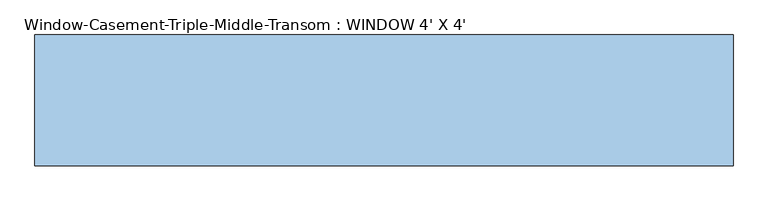
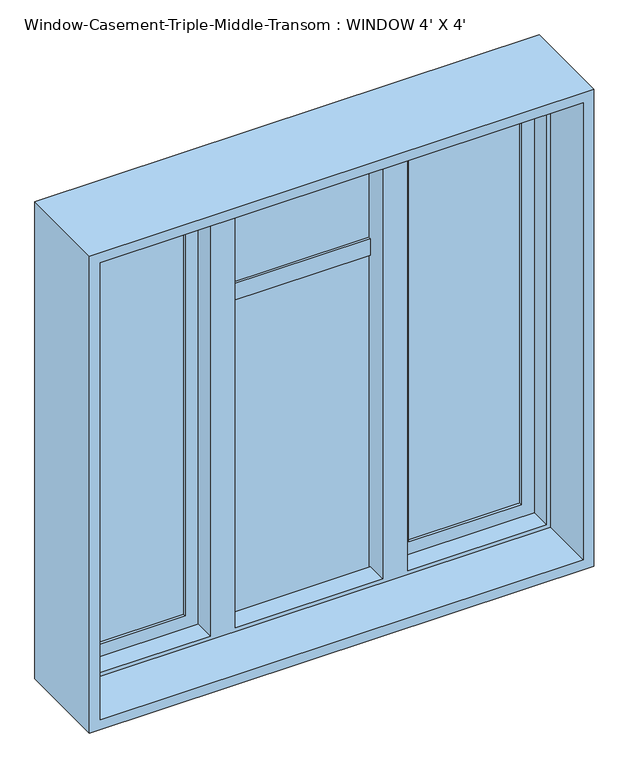
"""IFC4 building model written with IfcOpenShell, lengths in millimetres: window geometry, Window-Casement-Triple-Middle-Transom : WINDOW 4' X 4'."""

from ifc_helpers import new_model, si_unit, frame, origin, place, context, project, spatial, polyline, outline, extrude, faceted_brep, source, transform, mapped, element, save


def window_casement_triple_middle_transom_window_4_x_4_1416bf83(model_context):
    return source(origin(), model_context, "Body", "SolidModel", [
        extrude(outline(polyline([(2108.2, 228.6), (939.8, 228.6), (939.8, 584.2), (2108.2, 584.2), (2108.2, 228.6)]), holes=[polyline([(2066.3296875, 542.3296875), (981.6703125, 542.3296875), (981.6703125, 270.4703125), (2066.3296875, 270.4703125), (2066.3296875, 542.3296875)])]), frame((0.0, 73.025, 0.0), z_axis=(0.0, 1.0, 0.0), x_axis=(0.0, 0.0, 1.0)), (0.0, 0.0, 1.0), 31.75),
        extrude(outline(polyline([(2108.2, -584.2), (939.8, -584.2), (939.8, -228.6), (2108.2, -228.6), (2108.2, -584.2)]), holes=[polyline([(2066.3296875, -270.4703125), (981.6703125, -270.4703125), (981.6703125, -542.3296875), (2066.3296875, -542.3296875), (2066.3296875, -270.4703125)])]), frame((0.0, 73.025, 0.0), z_axis=(0.0, 1.0, 0.0), x_axis=(0.0, 0.0, 1.0)), (0.0, 0.0, 1.0), 31.75),
        extrude(outline(polyline([(-270.4703125, 98.425), (-270.4703125, 92.075), (-542.3296875, 92.075), (-542.3296875, 98.425), (-270.4703125, 98.425)])), frame((0.0, 0.0, 949.9203125), z_axis=(0.0, 0.0, 1.0), x_axis=(1.0, 0.0, 0.0)), (0.0, 0.0, 1.0), 1148.159375),
        extrude(outline(polyline([(-270.4703125, 85.725), (-270.4703125, 79.375), (-542.3296875, 79.375), (-542.3296875, 85.725), (-270.4703125, 85.725)])), frame((0.0, 0.0, 949.9203125), z_axis=(0.0, 0.0, 1.0), x_axis=(1.0, 0.0, 0.0)), (0.0, 0.0, 1.0), 1148.159375),
        extrude(outline(polyline([(542.3296875, 98.425), (542.3296875, 92.075), (270.4703125, 92.075), (270.4703125, 98.425), (542.3296875, 98.425)])), frame((0.0, 0.0, 949.9203125), z_axis=(0.0, 0.0, 1.0), x_axis=(1.0, 0.0, 0.0)), (0.0, 0.0, 1.0), 1148.159375),
        extrude(outline(polyline([(542.3296875, 85.725), (542.3296875, 79.375), (270.4703125, 79.375), (270.4703125, 85.725), (542.3296875, 85.725)])), frame((0.0, 0.0, 949.9203125), z_axis=(0.0, 0.0, 1.0), x_axis=(1.0, 0.0, 0.0)), (0.0, 0.0, 1.0), 1148.159375),
        extrude(outline(polyline([(177.8, 104.775), (177.8, 73.025), (-177.8, 73.025), (-177.8, 104.775), (177.8, 104.775)])), frame((0.0, 0.0, 1746.9048438), z_axis=(0.0, 0.0, 1.0), x_axis=(1.0, 0.0, 0.0)), (0.0, 0.0, 1.0), 41.8703125),
        extrude(outline(polyline([(177.8, 98.425), (177.8, 92.075), (-177.8, 92.075), (-177.8, 98.425), (177.8, 98.425)])), frame((0.0, 0.0, 939.8), z_axis=(0.0, 0.0, 1.0), x_axis=(1.0, 0.0, 0.0)), (0.0, 0.0, 1.0), 807.1048438),
        extrude(outline(polyline([(177.8, 85.725), (177.8, 79.375), (-177.8, 79.375), (-177.8, 85.725), (177.8, 85.725)])), frame((0.0, 0.0, 939.8), z_axis=(0.0, 0.0, 1.0), x_axis=(1.0, 0.0, 0.0)), (0.0, 0.0, 1.0), 807.1048438),
        extrude(outline(polyline([(177.8, 98.425), (177.8, 92.075), (-177.8, 92.075), (-177.8, 98.425), (177.8, 98.425)])), frame((0.0, 0.0, 1788.7751563), z_axis=(0.0, 0.0, 1.0), x_axis=(1.0, 0.0, 0.0)), (0.0, 0.0, 1.0), 319.4248438),
        extrude(outline(polyline([(177.8, 85.725), (177.8, 79.375), (-177.8, 79.375), (-177.8, 85.725), (177.8, 85.725)])), frame((0.0, 0.0, 1788.7751563), z_axis=(0.0, 0.0, 1.0), x_axis=(1.0, 0.0, 0.0)), (0.0, 0.0, 1.0), 319.4248438),
        faceted_brep([(-228.6, 73.025, 2108.2), (-584.2, 73.025, 2108.2), (-584.2, 114.3, 2108.2), (584.2, 114.3, 2108.2), (584.2, 73.025, 2108.2), (228.6, 73.025, 2108.2), (228.6, 111.125, 2108.2), (177.8, 111.125, 2108.2), (177.8, 73.025, 2108.2), (-177.8, 73.025, 2108.2), (-177.8, 111.125, 2108.2), (-228.6, 111.125, 2108.2), (-574.0796875, 22.225, 2098.0796875), (-574.0796875, 73.025, 2098.0796875), (-238.7203125, 73.025, 2098.0796875), (-238.7203125, 22.225, 2098.0796875), (574.0796875, 73.025, 2098.0796875), (574.0796875, 22.225, 2098.0796875), (238.7203125, 22.225, 2098.0796875), (238.7203125, 73.025, 2098.0796875), (-177.8, 73.025, 2098.0796875), (177.8, 73.025, 2098.0796875), (177.8, 22.225, 2098.0796875), (-177.8, 22.225, 2098.0796875), (-584.2, -114.3, 2108.2), (-584.2, 22.225, 2108.2), (584.2, 22.225, 2108.2), (584.2, -114.3, 2108.2), (-609.6, 114.3, 2133.6), (-609.6, -114.3, 2133.6), (609.6, -114.3, 2133.6), (609.6, 114.3, 2133.6), (584.2, 114.3, 939.8), (584.2, 73.025, 939.8), (574.0796875, 73.025, 949.9203125), (574.0796875, 22.225, 949.9203125), (584.2, 22.225, 939.8), (584.2, -114.3, 939.8), (609.6, -114.3, 914.4), (609.6, 114.3, 914.4), (228.6, 73.025, 939.8), (-584.2, 114.3, 939.8), (-584.2, 73.025, 939.8), (-228.6, 73.025, 939.8), (-228.6, 111.125, 939.8), (-177.8, 111.125, 939.8), (-177.8, 73.025, 939.8), (177.8, 73.025, 939.8), (177.8, 111.125, 939.8), (228.6, 111.125, 939.8), (238.7203125, 73.025, 949.9203125), (238.7203125, 22.225, 949.9203125), (-574.0796875, 73.025, 949.9203125), (-574.0796875, 22.225, 949.9203125), (-238.7203125, 22.225, 949.9203125), (-238.7203125, 73.025, 949.9203125), (177.8, 73.025, 949.9203125), (-177.8, 73.025, 949.9203125), (-177.8, 22.225, 949.9203125), (177.8, 22.225, 949.9203125), (-584.2, 22.225, 939.8), (-584.2, -114.3, 939.8), (-609.6, -114.3, 914.4), (-609.6, 114.3, 914.4)], [[[0, 1, 2, 3, 4, 5, 6, 7, 8, 9, 10, 11]], [[12, 13, 14, 15]], [[16, 17, 18, 19]], [[20, 21, 22, 23]], [[24, 25, 26, 27]], [[28, 29, 30, 31]], [[4, 3, 32, 33]], [[17, 16, 34, 35]], [[27, 26, 36, 37]], [[31, 30, 38, 39]], [[40, 33, 32, 41, 42, 43, 44, 45, 46, 47, 48, 49]], [[35, 34, 50, 51]], [[52, 53, 54, 55]], [[56, 57, 58, 59]], [[37, 36, 60, 61]], [[39, 38, 62, 63]], [[2, 1, 42, 41]], [[4, 33, 40, 5], [16, 19, 50, 34]], [[57, 56, 47, 46]], [[42, 1, 0, 43], [52, 55, 14, 13]], [[21, 20, 9, 8]], [[13, 12, 53, 52]], [[25, 24, 61, 60]], [[30, 29, 62, 38], [24, 27, 37, 61]], [[29, 28, 63, 62]], [[28, 31, 39, 63], [3, 2, 41, 32]], [[10, 45, 44, 11]], [[11, 44, 43, 0]], [[45, 10, 9, 20, 23, 58, 57, 46]], [[6, 49, 48, 7]], [[7, 48, 47, 56, 59, 22, 21, 8]], [[49, 6, 5, 40]], [[14, 55, 54, 15]], [[50, 19, 18, 51]], [[36, 26, 25, 60], [17, 35, 51, 18], [12, 15, 54, 53], [23, 22, 59, 58]]]),
    ])


if __name__ == "__main__":
    model = new_model("IFC4")
    model_context = context("Model", 3, world=origin())
    ifc_project = project(units=[si_unit("LENGTHUNIT", "METRE", prefix="MILLI")], contexts=[model_context])
    site = spatial("IfcSite", under=ifc_project)
    building = spatial("IfcBuilding", under=site)
    placement = place(None, origin())
    window_casement_triple_middle_transom_window_4_x_4_shape = window_casement_triple_middle_transom_window_4_x_4_1416bf83(model_context)
    element("IfcWindow", 1, ObjectType="Window-Casement-Triple-Middle-Transom : WINDOW 4' X 4'", at=placement, inside=building, context=model_context, shape_type="MappedRepresentation", body=[
        mapped(window_casement_triple_middle_transom_window_4_x_4_shape, transform((0.0, 0.0, 0.0), x_axis=(1.0, 0.0, 0.0), y_axis=(0.0, 1.0, 0.0), z_axis=(0.0, 0.0, 1.0))),
    ])
    save(model, "model.ifc")

# Revit data of these elements
# Type "Window-Casement-Triple-Middle-Transom : WINDOW 4' X 4'"
#   Type Mark = "21"
#   Fire Rating = "0.5h"
#   Assembly Code = "B2020100"
#   Analytic Construction = "Double glazing - domestic"
#   Window Width = 1' - 4"
#   Window Inset [instance default] = 0' - 0 5/8"
#   Wall Thickness [instance default] = 0' - 6"
#   Visual Light Transmittance = 0.81
#   Transom Height Ratio = 0.3
#   Thermal Resistance (R) = 1.8146 (h·ft²·°F)/BTU
#   Solar Heat Gain Coefficient = 0.76
#   Rough Width = 4' - 0 1/2"
#   Rough Height = 4' - 0 1/2"
#   Heat Transfer Coefficient (U) = 0.5511 BTU/(h·ft²·°F)
#   Height = 4' - 0"
#   Transom Height = 1' - 2.4"
#   Frame Gap 3 [instance default] = 0' - 1 83/128"
#   Frame Gap 2 [instance default] = 0' - 0 5/8"
#   Frame Gap 1 = 0' - 1 51/128"
#   Default Sill Height = 3' - 0"
#   Width = 4' - 0"
#   Frame Material = WOOD MATERIAL
#   Glass Panel Material = GLASS MATERIAL
#   Wall Closure = (empty or 0)
# Element 1 (IfcWindow, "Window-Casement-Triple-Middle-Transom : WINDOW 4' X 4'")
#   Wall Thickness = 0' - 9"
#   Materials on its faces: "WOOD MATERIAL", "GLASS MATERIAL"
# Materials
#   "WOOD MATERIAL": class "Generic", colour RGB 120 120 120, transparency 0, Cost = 0
#   "GLASS MATERIAL": class "Generic", colour RGB 120 120 120, transparency 0, Cost = 0
